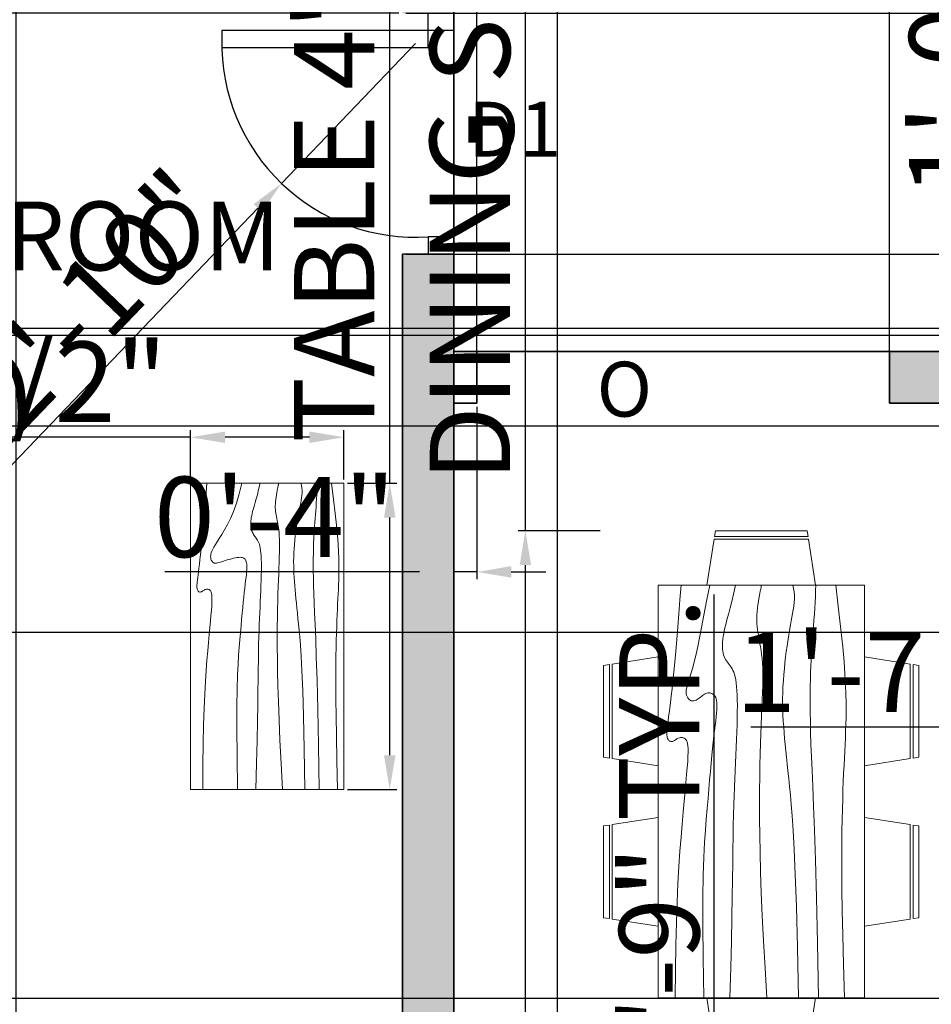
# Model space of a CAD drawing. Units: inches. Extents: x 2961 to 3748, y 1432 to 1961.
# Tile 3 of 9: x 3188 to 3348, y 1541 to 1713. Entities that reach past the tile are written whole.
import ezdxf
from ezdxf.enums import TextEntityAlignment as Align

# ---------------------------------------------------------------- set-up
doc = ezdxf.new("R2010")
doc.units = ezdxf.units.IN
for name, color, linetype, lineweight in [('A-ANNO-DIMS', 2, 'Continuous', 18), ('A-ANNO-TEXT', 7, 'Continuous', 18), ('A-AREA-IDEN', 7, 'Continuous', 18), ('A-DOOR', 3, 'Continuous', 25), ('A-FURN', 8, 'Continuous', 18), ('A-WALL', 7, 'Continuous', 35), ('A-WALL-PATT', 252, 'Continuous', 13)]:
    doc.layers.add(name, color=color, linetype=linetype, lineweight=lineweight)
doc.styles.get("Standard").update_dxf_attribs({"font": 'arial.ttf'})
doc.dimstyles.new('ISO-25', dxfattribs={"dimtxt": 14, "dimasz": 6, "dimexe": 1.25, "dimexo": 0.625, "dimtad": 1, "dimlunit": 3, "dimtxsty": 'Standard', "dimcen": 2.5, "dimadec": 0, "dimazin": 0, "dimtfac": 1, "dimtmove": 0, "dimatfit": 3, "dimfxl": 1, "dimarcsym": 0})

# ---------------------------------------------------------------- blocks, each defined once
blk = doc.blocks.new('Dining Set - 36 x 72 in.')
for p, q in [((-22, 27.5), (-22.1562, 26.50042)), ((-22, 27.5), (-6, 27.5)), ((-5.8437, 26.49966), (-6, 27.5)), ((6, 27.5), (5.8438, 26.50042)), ((6, 27.5), (22, 27.5)), ((22.1563, 26.49966), (22, 27.5)), ((-22.2343, 26.00059), (-23.4847, 17.99762)), ((-22.2304, 26), (-5.7608, 26)), ((-5.8416, 26.5), (-22.1534, 26.5)), ((-4.5152, 17.99762), (-5.7655, 25.99926)), ((5.7657, 26.00059), (4.5153, 17.99762)), ((5.7696, 26), (22.2392, 26)), ((22.1584, 26.5), (5.8466, 26.5)), ((23.4848, 17.99762), (22.2345, 25.99926)), ((36, 18), (-36, 18)), ((-36, 18), (-36, -18)), ((36, -18), (36, 18)), ((-44.0006, 8.23428), (-35.9976, 9.48474)), ((44.0006, 8.23428), (35.9976, 9.48474)), ((-45.5, 8), (-44.5004, 8.15617)), ((-45.5, 8), (-45.5, -8)), ((-44.5, -8.15843), (-44.5, 8.15338)), ((-44, 8.23041), (-44, -8.23915)), ((44, 8.23041), (44, -8.23915)), ((44.5, -8.15843), (44.5, 8.15338)), ((45.5, 8), (44.5005, 8.15617)), ((45.5, 8), (45.5, -8)), ((-44.4997, -8.15631), (-45.5, -8)), ((-35.9976, -9.48476), (-43.9993, -8.2345)), ((35.9976, -9.48476), (43.9993, -8.2345)), ((44.4997, -8.15631), (45.5, -8)), ((-36, -18), (36, -18)), ((-22.2343, -26.0006), (-23.4847, -17.99762)), ((-4.5152, -17.99762), (-5.7655, -25.99928)), ((5.7657, -26.0006), (4.5153, -17.99762)), ((23.4848, -17.99762), (22.2345, -25.99928)), ((-22.2304, -26), (-5.7608, -26)), ((-22, -27.5), (-22.1562, -26.50044)), ((-5.8416, -26.5), (-22.1534, -26.5)), ((-5.8437, -26.49967), (-6, -27.5)), ((5.7696, -26), (22.2392, -26)), ((6, -27.5), (5.8438, -26.50044)), ((22.1584, -26.5), (5.8466, -26.5)), ((22.1563, -26.49967), (22, -27.5)), ((-22, -27.5), (-6, -27.5)), ((6, -27.5), (22, -27.5))]:
    blk.add_line(p, q)
for points in [[(-36, 15), (-31.1772, 14.97754), (-26.8079, 14.91406), (-22.8538, 14.81543), (-19.276, 14.6875), (-16.0362, 14.53613), (-13.0957, 14.36718), (-10.4159, 14.18652), (-7.9583, 14), (-5.6904, 13.81315), (-3.6035, 13.63021), (-1.6954, 13.45508), (0.0365, 13.29166), (1.5945, 13.14388), (2.9811, 13.01562), (4.1988, 12.9108), (5.25, 12.83333), (6.1393, 12.78613), (6.8802, 12.76823), (7.4883, 12.77767), (7.9792, 12.8125), (8.3685, 12.87077), (8.6719, 12.95052), (8.9049, 13.0498), (9.0833, 13.16666), (9.2205, 13.29899), (9.3216, 13.44401), (9.3895, 13.59879), (9.4271, 13.76041), (9.4373, 13.92594), (9.4232, 14.09245), (9.3875, 14.257), (9.3333, 14.41666), (9.2638, 14.56917), (9.1836, 14.71484), (9.0975, 14.85465), (9.0104, 14.98958), (8.9272, 15.1206), (8.8529, 15.2487), (8.7922, 15.37483), (8.75, 15.5), (8.7305, 15.62467), (8.7344, 15.74739), (8.7617, 15.86621), (8.8125, 15.97916), (8.8867, 16.08431), (8.9844, 16.17968), (9.1055, 16.26334), (9.25, 16.33333), (9.4189, 16.38802), (9.6172, 16.42708), (9.8506, 16.45052), (10.125, 16.45833), (10.4463, 16.45052), (10.8203, 16.42708), (11.2529, 16.38802), (11.75, 16.33333), (12.3184, 16.26318), (12.9694, 16.17838), (13.7151, 16.07991), (14.5677, 15.96875), (15.5395, 15.84586), (16.6426, 15.71224), (17.8893, 15.56884), (19.2917, 15.41666), (20.859, 15.25667), (22.5879, 15.08984), (24.4721, 14.91715), (26.5052, 14.73958), (28.6809, 14.5581), (30.9929, 14.3737), (33.4347, 14.18733), (36, 14)], [(-36, 10), (-28.9766, 10.14274), (-23.1725, 10.20442), (-18.4241, 10.19775), (-14.5677, 10.13541), (-11.4399, 10.03011), (-8.877, 9.89453), (-6.7154, 9.74137), (-4.7917, 9.58333), (-2.9698, 9.43082), (-1.2246, 9.28515), (0.4415, 9.14534), (2.026, 9.01041), (3.5266, 8.87939), (4.9408, 8.7513), (6.266, 8.62516), (7.5, 8.5), (8.6411, 8.37549), (9.6914, 8.2539), (10.6538, 8.13818), (11.5312, 8.03125), (12.3267, 7.93603), (13.043, 7.85547), (13.6831, 7.79248), (14.25, 7.75), (14.7471, 7.7303), (15.1797, 7.73307), (15.5537, 7.75732), (15.875, 7.80208), (16.1494, 7.86637), (16.3828, 7.94922), (16.5811, 8.04964), (16.75, 8.16666), (16.8944, 8.29915), (17.0143, 8.44531), (17.1089, 8.60319), (17.1771, 8.77083), (17.218, 8.94629), (17.2305, 9.1276), (17.2137, 9.31282), (17.1667, 9.5), (17.0895, 9.6875), (16.987, 9.875), (16.8649, 10.0625), (16.7292, 10.25), (16.5856, 10.4375), (16.4401, 10.625), (16.2985, 10.8125), (16.1667, 11), (16.05, 11.18733), (15.9518, 11.3737), (15.8752, 11.5581), (15.8229, 11.73958), (15.798, 11.91715), (15.8034, 12.08984), (15.842, 12.25667), (15.9167, 12.41666), (16.0295, 12.56836), (16.1784, 12.70833), (16.3605, 12.83268), (16.5729, 12.9375), (16.8127, 13.01888), (17.0768, 13.07291), (17.3625, 13.0957), (17.6667, 13.08333), (17.9894, 13.03312), (18.3418, 12.94726), (18.7382, 12.82918), (19.1927, 12.68229), (19.7195, 12.51001), (20.3327, 12.31575), (21.0465, 12.10294), (21.875, 11.875), (22.8357, 11.63354), (23.959, 11.37304), (25.2786, 11.08618), (26.8282, 10.76562), (28.6414, 10.40405), (30.752, 9.99414), (33.1936, 9.52856), (36, 9)], [(-36, 5.5), (-30.7157, 5.3348), (-26.069, 5.20963), (-21.9946, 5.11767), (-18.4271, 5.05208), (-15.3009, 5.00602), (-12.5508, 4.97265), (-10.1112, 4.94515), (-7.9167, 4.91666), (-5.909, 4.88167), (-4.0586, 4.83984), (-2.3429, 4.79215), (-0.7396, 4.73958), (0.7739, 4.6831), (2.22, 4.6237), (3.6213, 4.56233), (5, 4.5), (6.373, 4.43782), (7.7344, 4.3776), (9.0723, 4.32129), (10.375, 4.27083), (11.6309, 4.22819), (12.8281, 4.19531), (13.9551, 4.17415), (15, 4.16666), (15.954, 4.17448), (16.819, 4.19791), (17.6001, 4.23698), (18.3021, 4.29166), (18.9299, 4.36198), (19.4883, 4.44791), (19.9823, 4.54948), (20.4167, 4.66666), (20.7969, 4.79899), (21.1302, 4.94401), (21.4245, 5.09879), (21.6875, 5.26041), (21.9271, 5.42594), (22.1511, 5.59245), (22.3672, 5.757), (22.5834, 5.91666), (22.8065, 6.06868), (23.0404, 6.21093), (23.2879, 6.34147), (23.5521, 6.45833), (23.8358, 6.55957), (24.142, 6.64323), (24.4735, 6.70735), (24.8334, 6.75), (25.2235, 6.76969), (25.642, 6.76692), (26.0858, 6.74267), (26.5521, 6.69791), (27.0379, 6.63362), (27.5404, 6.55078), (28.0565, 6.45036), (28.5834, 6.33333), (29.1242, 6.19987), (29.7071, 6.04687), (30.3661, 5.87044), (31.1354, 5.66666), (32.0493, 5.43164), (33.142, 5.16146), (34.4475, 4.85221), (36, 4.5)], [(-36, -1), (-30.7915, -0.6591), (-26.0195, -0.38216), (-21.6519, -0.16284), (-17.6563, 0.00521), (-14.0005, 0.12833), (-10.6523, 0.21289), (-7.5796, 0.26522), (-4.75, 0.29166), (-2.134, 0.29793), (0.2878, 0.28711), (2.5317, 0.26163), (4.6146, 0.22396), (6.5529, 0.17651), (8.3633, 0.12174), (10.0623, 0.06209), (11.6667, 0), (13.1899, -0.06201), (14.6341, -0.1211), (15.9982, -0.17432), (17.2813, -0.21875), (18.4823, -0.25147), (19.6003, -0.26953), (20.6343, -0.27002), (21.5834, -0.25), (22.4481, -0.20768), (23.2357, -0.14584), (23.9549, -0.06836), (24.6146, 0.02083), (25.2235, 0.11784), (25.7904, 0.21875), (26.3241, 0.31966), (26.8334, 0.41666), (27.3265, 0.50618), (27.8099, 0.58593), (28.2894, 0.65397), (28.7709, 0.70833), (29.2601, 0.74707), (29.763, 0.76823), (30.2855, 0.76985), (30.8334, 0.75), (31.4088, 0.70784), (31.9994, 0.64713), (32.589, 0.57275), (33.1615, 0.48958), (33.7008, 0.4025), (34.1908, 0.3164), (34.6153, 0.23616), (34.9584, 0.16666), (35.2099, 0.11165), (35.3848, 0.07031), (35.504, 0.04069), (35.5886, 0.02083), (35.6594, 0.00879), (35.7377, 0.0026), (35.8442, 0.00032), (36, 0)], [(-36, -6.5), (-27.1843, -6.31267), (-20.084, -6.1263), (-14.469, -5.9419), (-10.1094, -5.76042), (-6.7752, -5.58285), (-4.2363, -5.41016), (-2.2629, -5.24333), (-0.625, -5.08334), (0.8708, -4.93099), (2.2715, -4.78646), (3.5872, -4.64974), (4.8281, -4.52084), (6.0046, -4.39974), (7.127, -4.28646), (8.2053, -4.18099), (9.25, -4.08334), (10.2705, -3.99382), (11.2734, -3.91407), (12.2647, -3.84603), (13.25, -3.79167), (14.2354, -3.75293), (15.2266, -3.73177), (16.2295, -3.73015), (17.25, -3.75), (18.2912, -3.79248), (19.3451, -3.85547), (20.4009, -3.93604), (21.4479, -4.03125), (22.4754, -4.13819), (23.4727, -4.25391), (24.4289, -4.37549), (25.3334, -4.5), (26.1785, -4.62492), (26.9694, -4.74935), (27.7145, -4.87281), (28.4219, -4.99479), (29.1, -5.11483), (29.7572, -5.23242), (30.4016, -5.34709), (31.0417, -5.45834), (31.6837, -5.56437), (32.3262, -5.65821), (32.9658, -5.73153), (33.599, -5.77604), (34.2224, -5.78345), (34.8327, -5.74545), (35.4264, -5.65373), (36, -5.5)], [(-36, -10), (-26.4022, -9.81299), (-18.4675, -9.62891), (-11.9839, -9.45069), (-6.7396, -9.28125), (-2.5226, -9.12354), (0.8789, -8.98047), (3.6769, -8.85498), (6.0833, -8.75), (8.2767, -8.66765), (10.3021, -8.60677), (12.1712, -8.56543), (13.8958, -8.54167), (15.4876, -8.53353), (16.9583, -8.53907), (18.3197, -8.55632), (19.5834, -8.58334), (20.7616, -8.61841), (21.8685, -8.66081), (22.9188, -8.71004), (23.9271, -8.76563), (24.9081, -8.82707), (25.8763, -8.89388), (26.8465, -8.96558), (27.8334, -9.04167), (28.8474, -9.12118), (29.8828, -9.20117), (30.93, -9.27824), (31.9792, -9.34896), (33.0205, -9.40991), (34.0443, -9.45768), (35.0407, -9.48885), (36, -9.5)], [(-36, -14.5), (-30.0881, -14.33513), (-25.0332, -14.21224), (-20.7312, -14.12647), (-17.0781, -14.07292), (-13.97, -14.04671), (-11.3027, -14.04297), (-8.9724, -14.05681), (-6.875, -14.08334), (-4.9224, -14.11833), (-3.0905, -14.16016), (-1.3709, -14.20785), (0.2448, -14.26042), (1.7647, -14.3169), (3.1973, -14.3763), (4.5507, -14.43767), (5.8333, -14.5), (7.0554, -14.5621), (8.235, -14.62175), (9.3922, -14.67652), (10.5469, -14.72396), (11.7192, -14.76164), (12.929, -14.78711), (14.1965, -14.79794), (15.5417, -14.79167), (16.9933, -14.76424), (18.6152, -14.70508), (20.4804, -14.60197), (22.6615, -14.44271), (25.2312, -14.21509), (28.2624, -13.9069), (31.8277, -13.50594), (36, -13)]]:
    blk.add_lwpolyline(points)
blk = doc.blocks.new('Table - Rectangular Woodgrain 60 x 30 in.')
for p, q in [((0, 0), (0, -30)), ((60, 0), (0, 0)), ((60, -30), (60, 0)), ((0, -30), (60, -30))]:
    blk.add_line(p, q)
for points in [[(0, -2.4), (4.8155, -2.418), (9.0302, -2.4688), (12.709, -2.5477), (15.9167, -2.65), (18.7181, -2.7711), (21.1781, -2.9063), (23.3616, -3.0508), (25.3333, -3.2), (27.1477, -3.3495), (28.8172, -3.4958), (30.3437, -3.636), (31.7291, -3.7667), (32.9756, -3.8849), (34.0849, -3.9875), (35.059, -4.0714), (35.9, -4.1334), (36.6114, -4.1711), (37.2041, -4.1854), (37.6906, -4.1779), (38.0833, -4.15), (38.3948, -4.1034), (38.6375, -4.0396), (38.8239, -3.9602), (38.9666, -3.8667), (39.0764, -3.7608), (39.1573, -3.6448), (39.2116, -3.521), (39.2416, -3.3917), (39.2498, -3.2593), (39.2385, -3.1261), (39.21, -2.9944), (39.1666, -2.8667), (39.111, -2.7447), (39.0468, -2.6281), (38.978, -2.5163), (38.9083, -2.4083), (38.8418, -2.3035), (38.7823, -2.201), (38.7337, -2.1001), (38.7, -2), (38.6844, -1.9003), (38.6875, -1.8021), (38.7094, -1.707), (38.75, -1.6167), (38.8094, -1.5326), (38.8875, -1.4563), (38.9844, -1.3893), (39.1, -1.3333), (39.2351, -1.2896), (39.3937, -1.2583), (39.5804, -1.2396), (39.8, -1.2333), (40.057, -1.2396), (40.3562, -1.2583), (40.7023, -1.2896), (41.1, -1.3333), (41.5547, -1.3895), (42.0755, -1.4573), (42.6721, -1.5361), (43.3542, -1.625), (44.1316, -1.7233), (45.014, -1.8302), (46.0114, -1.9449), (47.1333, -2.0667), (48.3862, -2.1947), (49.7625, -2.3281), (51.2513, -2.4663), (52.8416, -2.6083), (54.5226, -2.7535), (56.2833, -2.9011), (58.1127, -3.0501), (60, -3.2)], [(0, -9.2), (6.5759, -9.0858), (11.9385, -9.0365), (16.2527, -9.0418), (19.6833, -9.0917), (22.3952, -9.1759), (24.5531, -9.2844), (26.322, -9.4069), (27.8666, -9.5333), (29.3241, -9.6553), (30.7203, -9.7719), (32.0532, -9.8837), (33.3208, -9.9917), (34.5213, -10.0965), (35.6526, -10.199), (36.7128, -10.2999), (37.7, -10.4), (38.6129, -10.4996), (39.4531, -10.5969), (40.223, -10.6895), (40.925, -10.775), (41.5613, -10.8512), (42.1344, -10.9156), (42.6465, -10.966), (43.1, -11), (43.4976, -11.0158), (43.8437, -11.0136), (44.143, -10.9942), (44.4, -10.9583), (44.6195, -10.9069), (44.8062, -10.8406), (44.9648, -10.7603), (45.1, -10.6667), (45.2155, -10.5598), (45.3114, -10.4365), (45.3871, -10.2929), (45.4416, -10.125), (45.4743, -9.929), (45.4844, -9.7011), (45.4709, -9.4371), (45.4333, -9.1333), (45.3716, -8.7883), (45.2896, -8.4104), (45.1919, -8.0107), (45.0833, -7.6), (44.9685, -7.1893), (44.8521, -6.7896), (44.7388, -6.4117), (44.6333, -6.0667), (44.54, -5.7628), (44.4614, -5.4979), (44.4001, -5.2675), (44.3583, -5.0667), (44.3384, -4.8909), (44.3427, -4.7354), (44.3736, -4.5956), (44.4333, -4.4667), (44.5236, -4.3453), (44.6427, -4.2333), (44.7884, -4.1339), (44.9583, -4.05), (45.1501, -3.9849), (45.3614, -3.9417), (45.59, -3.9234), (45.8333, -3.9333), (46.0915, -3.9749), (46.3734, -4.0531), (46.6906, -4.1736), (47.0542, -4.3417), (47.4756, -4.5629), (47.9661, -4.8427), (48.5372, -5.1866), (49.2, -5.6), (49.9676, -6.0844), (50.8594, -6.625), (51.8965, -7.2031), (53.1, -7.8), (54.491, -8.3969), (56.0906, -8.975), (57.9199, -9.5156), (60, -10)], [(0, -12.8), (5.1847, -12.9322), (9.6213, -13.0323), (13.3963, -13.1059), (16.5958, -13.1583), (19.3063, -13.1952), (21.614, -13.2219), (23.6054, -13.2439), (25.3666, -13.2667), (26.9728, -13.2947), (28.4531, -13.3281), (29.8256, -13.3663), (31.1083, -13.4083), (32.3191, -13.4535), (33.476, -13.501), (34.597, -13.5501), (35.7, -13.6), (36.7984, -13.6497), (37.8875, -13.6979), (38.9578, -13.743), (40, -13.7833), (41.0047, -13.8174), (41.9625, -13.8438), (42.864, -13.8607), (43.7, -13.8667), (44.4631, -13.8604), (45.1552, -13.8417), (45.7801, -13.8104), (46.3416, -13.7667), (46.8439, -13.7104), (47.2906, -13.6417), (47.6858, -13.5604), (48.0333, -13.4667), (48.3375, -13.3608), (48.6042, -13.2448), (48.8396, -13.121), (49.05, -12.9917), (49.2417, -12.8593), (49.4208, -12.7261), (49.5937, -12.5944), (49.7667, -12.4667), (49.9452, -12.3451), (50.1323, -12.2313), (50.3303, -12.1268), (50.5416, -12.0333), (50.7686, -11.9524), (51.0135, -11.8854), (51.2788, -11.8341), (51.5666, -11.8), (51.8785, -11.7843), (52.2116, -11.7865), (52.562, -11.8059), (52.926, -11.8417), (53.2998, -11.8931), (53.6795, -11.9594), (54.0614, -12.0397), (54.4416, -12.1333), (54.8223, -12.2401), (55.2293, -12.3625), (55.6942, -12.5037), (56.2489, -12.6667), (56.9251, -12.8547), (57.7545, -13.0708), (58.7689, -13.3182), (60, -13.6)], [(0, -18), (5.124, -17.7273), (9.6609, -17.5057), (13.6705, -17.3303), (17.2125, -17.1958), (20.3467, -17.0973), (23.1328, -17.0297), (25.6307, -16.9878), (27.9, -16.9667), (29.9928, -16.9617), (31.9302, -16.9703), (33.7254, -16.9907), (35.3917, -17.0208), (36.9423, -17.0588), (38.3906, -17.1026), (39.7499, -17.1503), (41.0333, -17.2), (42.2519, -17.2496), (43.4073, -17.2969), (44.4986, -17.3395), (45.525, -17.375), (46.4858, -17.4012), (47.3802, -17.4156), (48.2074, -17.416), (48.9667, -17.4), (49.6583, -17.3662), (50.2872, -17.3167), (50.8595, -17.2547), (51.3812, -17.1833), (51.8584, -17.1057), (52.2971, -17.025), (52.7034, -16.9443), (53.0833, -16.8667), (53.443, -16.7951), (53.789, -16.7313), (54.128, -16.6768), (54.4666, -16.6334), (54.8115, -16.6024), (55.1693, -16.5854), (55.5465, -16.5841), (55.95, -16.6), (56.3828, -16.6337), (56.8346, -16.6823), (57.2915, -16.7418), (57.7396, -16.8084), (58.165, -16.878), (58.5539, -16.9469), (58.8924, -17.0111), (59.1666, -17.0667), (59.3679, -17.1107), (59.5078, -17.1438), (59.6032, -17.1675), (59.6708, -17.1833), (59.7275, -17.193), (59.7901, -17.1979), (59.8753, -17.1998), (60, -17.2)], [(0, -22.4), (8.0098, -22.2501), (14.4094, -22.1011), (19.4168, -21.9535), (23.25, -21.8083), (26.1269, -21.6663), (28.2656, -21.5281), (29.884, -21.3947), (31.2, -21.2667), (32.3967, -21.1448), (33.5172, -21.0292), (34.5697, -20.9198), (35.5625, -20.8167), (36.5037, -20.7198), (37.4015, -20.6292), (38.2642, -20.5448), (39.1, -20.4667), (39.9164, -20.3951), (40.7187, -20.3313), (41.5117, -20.2768), (42.3, -20.2333), (43.0883, -20.2024), (43.8812, -20.1854), (44.6836, -20.1841), (45.5, -20.2), (46.3328, -20.234), (47.1747, -20.2844), (48.0163, -20.3488), (48.8479, -20.425), (49.66, -20.5106), (50.4429, -20.6031), (51.1872, -20.7004), (51.8833, -20.8), (52.5246, -20.8999), (53.1166, -20.9995), (53.6681, -21.0983), (54.1875, -21.1958), (54.6834, -21.2919), (55.1646, -21.3859), (55.6394, -21.4777), (56.1167, -21.5667), (56.6028, -21.6515), (57.0961, -21.7266), (57.5929, -21.7852), (58.0896, -21.8208), (58.5823, -21.8268), (59.0674, -21.7964), (59.5412, -21.723), (60, -21.6)], [(0, -25.2), (8.6355, -25.0504), (15.7026, -24.9031), (21.4049, -24.7606), (25.9458, -24.625), (29.529, -24.4988), (32.3578, -24.3844), (34.6359, -24.284), (36.5667, -24.2), (38.3213, -24.1341), (39.9417, -24.0854), (41.437, -24.0523), (42.8167, -24.0333), (44.0901, -24.0268), (45.2667, -24.0313), (46.3557, -24.0451), (47.3667, -24.0667), (48.309, -24.0947), (49.1928, -24.1287), (50.0284, -24.168), (50.826, -24.2125), (51.5959, -24.2617), (52.3483, -24.3151), (53.0935, -24.3725), (53.8417, -24.4334), (54.6009, -24.497), (55.3699, -24.561), (56.1454, -24.6226), (56.9239, -24.6792), (57.7021, -24.7279), (58.4764, -24.7662), (59.2435, -24.7911), (60, -24.8)], [(0, -28.8), (5.6867, -28.6681), (10.45, -28.5698), (14.407, -28.5012), (17.675, -28.4584), (20.3711, -28.4374), (22.6125, -28.4344), (24.5164, -28.4455), (26.2, -28.4667), (27.762, -28.4947), (29.2276, -28.5281), (30.6033, -28.5663), (31.8958, -28.6084), (33.1118, -28.6535), (34.2578, -28.7011), (35.3405, -28.7501), (36.3666, -28.8), (37.3443, -28.8497), (38.288, -28.8974), (39.2137, -28.9412), (40.1375, -28.9792), (41.0753, -29.0093), (42.0432, -29.0297), (43.0572, -29.0384), (44.1333, -29.0333), (45.2936, -29.0114), (46.5843, -28.9641), (48.0579, -28.8816), (49.7666, -28.7542), (51.7629, -28.5721), (54.0989, -28.3255), (56.8272, -28.0048), (60, -27.6)]]:
    blk.add_lwpolyline(points)
blk = doc.blocks.new('*D21')
at = {"layer": 'A-ANNO-DIMS', "color": 0, "lineweight": -2, "transparency": 16777216}
for p, q in [((3309.67, 1519.64), (3309.67, 1612.23)), ((3304.89, 1513.64), (3310.92, 1513.64)), ((3309.67, 1504.64), (3309.67, 1513.64)), ((3304.89, 1504.64), (3310.92, 1504.64)), ((3309.67, 1498.64), (3309.67, 1492.64))]:
    blk.add_line(p, q, dxfattribs=at)
at = {"layer": 'A-ANNO-DIMS', "color": 0, "transparency": 16777216}
for points in [[(3308.67, 1519.64), (3310.67, 1519.64), (3309.67, 1513.64)], [(3308.67, 1498.64), (3310.67, 1498.64), (3309.67, 1504.64)]]:
    blk.add_solid(points, dxfattribs=at)
at = {"layer": 'Defpoints', "color": 0, "transparency": 16777216}
for p in [(3304.27, 1513.64), (3309.67, 1513.64), (3304.27, 1504.64)]:
    blk.add_point(p, dxfattribs=at)
at = {"layer": 'A-ANNO-DIMS', "color": 0, "transparency": 16777216, "insert": (3301.89, 1568.93), "char_height": 14, "attachment_point": 5, "rotation": 90}
blk.add_mtext('0\'-9" TYP.', dxfattribs=at)
blk = doc.blocks.new('*D28')
at = {"layer": 'A-ANNO-DIMS', "color": 0, "lineweight": -2, "transparency": 16777216}
for p, q in [((3253.06, 1631.67), (3253.06, 1776.5)), ((3245.67, 1631.67), (3254.31, 1631.67)), ((3253.06, 1584.22), (3253.06, 1625.67)), ((3245.67, 1578.22), (3254.31, 1578.22))]:
    blk.add_line(p, q, dxfattribs=at)
at = {"layer": 'A-ANNO-DIMS', "color": 0, "transparency": 16777216}
for points in [[(3252.06, 1625.67), (3254.06, 1625.67), (3253.06, 1631.67)], [(3252.06, 1584.22), (3254.06, 1584.22), (3253.06, 1578.22)]]:
    blk.add_solid(points, dxfattribs=at)
at = {"layer": 'Defpoints', "color": 0, "transparency": 16777216}
for p in [(3245.04, 1631.67), (3253.06, 1631.67), (3245.04, 1578.22)]:
    blk.add_point(p, dxfattribs=at)
at = {"layer": 'A-ANNO-DIMS', "color": 0, "transparency": 16777216, "insert": (3245.19, 1707.08), "char_height": 14, "attachment_point": 5, "rotation": 90}
blk.add_mtext('TABLE 4\'-5 1/2"', dxfattribs=at)
blk = doc.blocks.new('*D29')
at = {"layer": 'A-ANNO-DIMS', "color": 0, "lineweight": -2, "transparency": 16777216}
for p, q in [((3218.32, 1632.29), (3218.32, 1640.93)), ((3245.04, 1632.29), (3245.04, 1640.93)), ((3218.32, 1639.68), (3140.99, 1639.68)), ((3239.04, 1639.68), (3224.32, 1639.68))]:
    blk.add_line(p, q, dxfattribs=at)
at = {"layer": 'A-ANNO-DIMS', "color": 0, "transparency": 16777216}
for points in [[(3224.32, 1640.68), (3224.32, 1638.68), (3218.32, 1639.68)], [(3239.04, 1640.68), (3239.04, 1638.68), (3245.04, 1639.68)]]:
    blk.add_solid(points, dxfattribs=at)
at = {"layer": 'Defpoints', "color": 0, "transparency": 16777216}
for p in [(3218.32, 1639.68), (3218.32, 1631.67), (3245.04, 1631.67)]:
    blk.add_point(p, dxfattribs=at)
at = {"layer": 'A-ANNO-DIMS', "color": 0, "transparency": 16777216, "insert": (3176.66, 1647.55), "char_height": 14, "attachment_point": 5}
blk.add_mtext('2\'-2 1/2"', dxfattribs=at)
blk = doc.blocks.new('*D41')
at = {"layer": 'A-ANNO-DIMS', "color": 0, "lineweight": -2, "transparency": 16777216}
for p, q in [((3391.84, 1586.08), (3391.84, 1590.35)), ((3411.44, 1586.08), (3411.44, 1590.35)), ((3391.84, 1589.1), (3316.07, 1589.1)), ((3405.44, 1589.1), (3397.84, 1589.1))]:
    blk.add_line(p, q, dxfattribs=at)
at = {"layer": 'A-ANNO-DIMS', "color": 0, "transparency": 16777216}
for points in [[(3397.84, 1590.1), (3397.84, 1588.1), (3391.84, 1589.1)], [(3405.44, 1590.1), (3405.44, 1588.1), (3411.44, 1589.1)]]:
    blk.add_solid(points, dxfattribs=at)
at = {"layer": 'Defpoints', "color": 0, "transparency": 16777216}
for p in [(3391.84, 1589.1), (3391.84, 1585.45), (3411.44, 1585.45)]:
    blk.add_point(p, dxfattribs=at)
at = {"layer": 'A-ANNO-DIMS', "color": 0, "transparency": 16777216, "insert": (3350.95, 1596.96), "char_height": 14, "attachment_point": 5}
blk.add_mtext('1\'-7 1/2"', dxfattribs=at)
blk = doc.blocks.new('*D44')
at = {"layer": 'A-ANNO-DIMS', "color": 0, "lineweight": -2, "transparency": 16777216}
for p, q in [((3276.73, 1623.38), (3276.73, 1784.51)), ((3289.75, 1623.38), (3275.48, 1623.38)), ((3276.73, 1538.38), (3276.73, 1617.38)), ((3289.75, 1532.38), (3275.48, 1532.38))]:
    blk.add_line(p, q, dxfattribs=at)
at = {"layer": 'A-ANNO-DIMS', "color": 0, "transparency": 16777216}
for points in [[(3275.73, 1617.38), (3277.73, 1617.38), (3276.73, 1623.38)], [(3275.73, 1538.38), (3277.73, 1538.38), (3276.73, 1532.38)]]:
    blk.add_solid(points, dxfattribs=at)
at = {"layer": 'Defpoints', "color": 0, "transparency": 16777216}
for p in [(3276.73, 1623.38), (3290.38, 1623.38), (3290.38, 1532.38)]:
    blk.add_point(p, dxfattribs=at)
at = {"layer": 'A-ANNO-DIMS', "color": 0, "transparency": 16777216, "insert": (3268.87, 1706.94), "char_height": 14, "attachment_point": 5, "rotation": 90}
blk.add_mtext('DINING SET 7\'-7"', dxfattribs=at)
blk = doc.blocks.new('*D52')
at = {"layer": 'A-ANNO-DIMS', "color": 0, "lineweight": -2, "transparency": 16777216}
for p, q in [((3360.27, 1678.21), (3360.27, 1721.36)), ((3389.1, 1672.21), (3359.02, 1672.21)), ((3360.27, 1660.05), (3360.27, 1672.21)), ((3389.1, 1660.05), (3359.02, 1660.05)), ((3360.27, 1654.05), (3360.27, 1648.05))]:
    blk.add_line(p, q, dxfattribs=at)
at = {"layer": 'A-ANNO-DIMS', "color": 0, "transparency": 16777216}
for points in [[(3359.27, 1678.21), (3361.27, 1678.21), (3360.27, 1672.21)], [(3359.27, 1654.05), (3361.27, 1654.05), (3360.27, 1660.05)]]:
    blk.add_solid(points, dxfattribs=at)
at = {"layer": 'Defpoints', "color": 0, "transparency": 16777216}
for p in [(3360.27, 1672.21), (3389.72, 1672.21), (3389.72, 1660.05)]:
    blk.add_point(p, dxfattribs=at)
at = {"layer": 'A-ANNO-DIMS', "color": 0, "transparency": 16777216, "insert": (3352.5, 1702.78), "char_height": 14, "attachment_point": 5, "rotation": 90}
blk.add_mtext('1\'-0"', dxfattribs=at)
blk = doc.blocks.new('*D53')
at = {"layer": 'A-ANNO-DIMS', "color": 0, "lineweight": -2, "transparency": 16777216}
for p, q in [((3123.27, 1855.01), (3123.27, 1473.94)), ((3187.8, 1855.01), (3187.8, 1473.94)), ((3129.27, 1475.19), (3181.8, 1475.19)), ((3187.8, 1475.19), (3264.89, 1475.19))]:
    blk.add_line(p, q, dxfattribs=at)
at = {"layer": 'A-ANNO-DIMS', "color": 0, "transparency": 16777216}
for points in [[(3129.27, 1476.19), (3129.27, 1474.19), (3123.27, 1475.19)], [(3181.8, 1476.19), (3181.8, 1474.19), (3187.8, 1475.19)]]:
    blk.add_solid(points, dxfattribs=at)
at = {"layer": 'Defpoints', "color": 0, "transparency": 16777216}
for p in [(3123.27, 1855.64), (3187.8, 1855.64), (3187.8, 1475.19)]:
    blk.add_point(p, dxfattribs=at)
at = {"layer": 'A-ANNO-DIMS', "color": 0, "transparency": 16777216, "insert": (3229.35, 1483.05), "char_height": 14, "attachment_point": 5}
blk.add_mtext('5\'-4 1/2"', dxfattribs=at)
blk = doc.blocks.new('*D68')
at = {"layer": 'A-ANNO-DIMS', "color": 0, "lineweight": -2, "transparency": 16777216}
for p, q in [((3024.82, 1658.64), (3024.82, 1701.79)), ((3509.64, 1658.64), (3023.57, 1658.64)), ((3024.82, 1647.64), (3024.82, 1652.64)), ((3509.64, 1641.64), (3023.57, 1641.64))]:
    blk.add_line(p, q, dxfattribs=at)
at = {"layer": 'A-ANNO-DIMS', "color": 0, "transparency": 16777216}
for points in [[(3023.82, 1652.64), (3025.82, 1652.64), (3024.82, 1658.64)], [(3023.82, 1647.64), (3025.82, 1647.64), (3024.82, 1641.64)]]:
    blk.add_solid(points, dxfattribs=at)
at = {"layer": 'Defpoints', "color": 0, "transparency": 16777216}
for p in [(3024.82, 1658.64), (3510.27, 1658.64), (3510.27, 1641.64)]:
    blk.add_point(p, dxfattribs=at)
at = {"layer": 'A-ANNO-DIMS', "color": 0, "transparency": 16777216, "insert": (3017.04, 1683.21), "char_height": 14, "attachment_point": 5, "rotation": 90}
blk.add_mtext('1\'-5"', dxfattribs=at)
blk = doc.blocks.new('*D69')
at = {"layer": 'A-ANNO-DIMS', "color": 0, "lineweight": -2, "transparency": 16777216}
for p, q in [((3268.27, 1646.26), (3268.27, 1933.63)), ((3274.27, 1932.38), (3334.27, 1932.38)), ((3340.27, 1646.26), (3340.27, 1933.63))]:
    blk.add_line(p, q, dxfattribs=at)
at = {"layer": 'A-ANNO-DIMS', "color": 0, "transparency": 16777216}
for points in [[(3274.27, 1933.38), (3274.27, 1931.38), (3268.27, 1932.38)], [(3334.27, 1933.38), (3334.27, 1931.38), (3340.27, 1932.38)]]:
    blk.add_solid(points, dxfattribs=at)
at = {"layer": 'Defpoints', "color": 0, "transparency": 16777216}
for p in [(3340.27, 1932.38), (3268.27, 1645.64), (3340.27, 1645.64)]:
    blk.add_point(p, dxfattribs=at)
at = {"layer": 'A-ANNO-DIMS', "color": 0, "transparency": 16777216, "insert": (3304.27, 1940.15), "char_height": 14, "attachment_point": 5}
blk.add_mtext('6\'-0"', dxfattribs=at)
blk = doc.blocks.new('*D70')
at = {"layer": 'A-ANNO-DIMS', "color": 0, "lineweight": -2, "transparency": 16777216}
for p, q in [((3024.82, 1641.64), (3024.82, 1686.09)), ((3383.64, 1641.64), (3023.57, 1641.64)), ((3024.82, 1611.64), (3024.82, 1635.64)), ((3383.64, 1605.64), (3023.57, 1605.64))]:
    blk.add_line(p, q, dxfattribs=at)
at = {"layer": 'A-ANNO-DIMS', "color": 0, "transparency": 16777216}
for points in [[(3023.82, 1635.64), (3025.82, 1635.64), (3024.82, 1641.64)], [(3023.82, 1611.64), (3025.82, 1611.64), (3024.82, 1605.64)]]:
    blk.add_solid(points, dxfattribs=at)
at = {"layer": 'Defpoints', "color": 0, "transparency": 16777216}
for p in [(3024.82, 1641.64), (3384.27, 1641.64), (3384.27, 1605.64)]:
    blk.add_point(p, dxfattribs=at)
at = {"layer": 'A-ANNO-DIMS', "color": 0, "transparency": 16777216, "insert": (3017.04, 1666.87), "char_height": 14, "attachment_point": 5, "rotation": 90}
blk.add_mtext('3\'-0"', dxfattribs=at)
blk = doc.blocks.new('*D72')
at = {"layer": 'A-ANNO-DIMS', "color": 0, "lineweight": -2, "transparency": 16777216}
for p, q in [((3255.89, 1713.64), (3633.97, 1713.64)), ((3632.72, 1677.64), (3632.72, 1707.64)), ((3255.89, 1671.64), (3633.97, 1671.64))]:
    blk.add_line(p, q, dxfattribs=at)
at = {"layer": 'A-ANNO-DIMS', "color": 0, "transparency": 16777216}
for points in [[(3631.72, 1707.64), (3633.72, 1707.64), (3632.72, 1713.64)], [(3631.72, 1677.64), (3633.72, 1677.64), (3632.72, 1671.64)]]:
    blk.add_solid(points, dxfattribs=at)
at = {"layer": 'Defpoints', "color": 0, "transparency": 16777216}
for p in [(3255.27, 1713.64), (3632.72, 1713.64), (3255.27, 1671.64)]:
    blk.add_point(p, dxfattribs=at)
at = {"layer": 'A-ANNO-DIMS', "color": 0, "transparency": 16777216, "insert": (3624.94, 1692.64), "char_height": 14, "attachment_point": 5, "rotation": 90}
blk.add_mtext('3\'-6"', dxfattribs=at)
blk = doc.blocks.new('*D75')
at = {"layer": 'A-ANNO-DIMS', "color": 0, "lineweight": -2, "transparency": 16777216}
for p, q in [((3024.82, 1723.64), (3024.82, 1729.64)), ((3254.64, 1717.64), (3023.57, 1717.64)), ((3024.82, 1717.64), (3024.82, 1713.64)), ((3254.64, 1713.64), (3023.57, 1713.64)), ((3024.82, 1707.64), (3024.82, 1663.17))]:
    blk.add_line(p, q, dxfattribs=at)
at = {"layer": 'A-ANNO-DIMS', "color": 0, "transparency": 16777216}
for points in [[(3023.82, 1723.64), (3025.82, 1723.64), (3024.82, 1717.64)], [(3023.82, 1707.64), (3025.82, 1707.64), (3024.82, 1713.64)]]:
    blk.add_solid(points, dxfattribs=at)
at = {"layer": 'Defpoints', "color": 0, "transparency": 16777216}
for p in [(3255.27, 1717.64), (3024.82, 1713.64), (3255.27, 1713.64)]:
    blk.add_point(p, dxfattribs=at)
at = {"layer": 'A-ANNO-DIMS', "color": 0, "transparency": 16777216, "insert": (3017.04, 1682.41), "char_height": 14, "attachment_point": 5, "rotation": 90}
blk.add_mtext('0\'-4"', dxfattribs=at)
blk = doc.blocks.new('*D77')
at = {"layer": 'A-ANNO-DIMS', "color": 0, "lineweight": -2, "transparency": 16777216}
for p, q in [((3264.27, 1775.91), (3264.27, 1473.94)), ((3282.27, 1775.91), (3282.27, 1473.94)), ((3270.27, 1475.19), (3276.27, 1475.19)), ((3282.27, 1475.19), (3325.41, 1475.19))]:
    blk.add_line(p, q, dxfattribs=at)
at = {"layer": 'A-ANNO-DIMS', "color": 0, "transparency": 16777216}
for points in [[(3270.27, 1476.19), (3270.27, 1474.19), (3264.27, 1475.19)], [(3276.27, 1476.19), (3276.27, 1474.19), (3282.27, 1475.19)]]:
    blk.add_solid(points, dxfattribs=at)
at = {"layer": 'Defpoints', "color": 0, "transparency": 16777216}
for p in [(3264.27, 1776.53), (3282.27, 1776.53), (3282.27, 1475.19)]:
    blk.add_point(p, dxfattribs=at)
at = {"layer": 'A-ANNO-DIMS', "color": 0, "transparency": 16777216, "insert": (3306.84, 1482.96), "char_height": 14, "attachment_point": 5}
blk.add_mtext('1\'-6"', dxfattribs=at)
blk = doc.blocks.new('*D81')
at = {"layer": 'A-ANNO-DIMS', "color": 0, "lineweight": -2, "transparency": 16777216}
for p, q in [((3063.89, 1657.48), (3633.97, 1657.48)), ((3632.72, 1547.87), (3632.72, 1651.48)), ((3063.89, 1541.87), (3633.97, 1541.87))]:
    blk.add_line(p, q, dxfattribs=at)
at = {"layer": 'A-ANNO-DIMS', "color": 0, "transparency": 16777216}
for points in [[(3631.72, 1651.48), (3633.72, 1651.48), (3632.72, 1657.48)], [(3631.72, 1547.87), (3633.72, 1547.87), (3632.72, 1541.87)]]:
    blk.add_solid(points, dxfattribs=at)
at = {"layer": 'Defpoints', "color": 0, "transparency": 16777216}
for p in [(3063.27, 1657.48), (3632.72, 1657.48), (3063.27, 1541.87)]:
    blk.add_point(p, dxfattribs=at)
at = {"layer": 'A-ANNO-DIMS', "color": 0, "transparency": 16777216, "insert": (3624.85, 1599.67), "char_height": 14, "attachment_point": 5, "rotation": 90}
blk.add_mtext('9\'-7 1/2"', dxfattribs=at)
blk = doc.blocks.new('*D84')
at = {"layer": 'A-ANNO-DIMS', "color": 0, "lineweight": -2, "transparency": 16777216}
for p, q in [((3123.27, 1855.01), (3123.27, 1473.94)), ((3137.88, 1855.01), (3137.88, 1473.94)), ((3129.27, 1475.19), (3131.88, 1475.19)), ((3137.88, 1475.19), (3213.65, 1475.19))]:
    blk.add_line(p, q, dxfattribs=at)
at = {"layer": 'A-ANNO-DIMS', "color": 0, "transparency": 16777216}
for points in [[(3129.27, 1476.19), (3129.27, 1474.19), (3123.27, 1475.19)], [(3131.88, 1476.19), (3131.88, 1474.19), (3137.88, 1475.19)]]:
    blk.add_solid(points, dxfattribs=at)
at = {"layer": 'Defpoints', "color": 0, "transparency": 16777216}
for p in [(3123.27, 1855.64), (3137.88, 1855.64), (3137.88, 1475.19)]:
    blk.add_point(p, dxfattribs=at)
at = {"layer": 'A-ANNO-DIMS', "color": 0, "transparency": 16777216, "insert": (3178.76, 1483.05), "char_height": 14, "attachment_point": 5}
blk.add_mtext('1\'-2 1/2"', dxfattribs=at)
blk = doc.blocks.new('*D89')
at = {"layer": 'A-ANNO-DIMS', "color": 0, "lineweight": -2, "transparency": 16777216}
for p, q in [((3264.27, 1645.01), (3264.27, 1614.94)), ((3268.27, 1645.01), (3268.27, 1614.94)), ((3258.27, 1616.19), (3213.8, 1616.19)), ((3268.27, 1616.19), (3264.27, 1616.19)), ((3274.27, 1616.19), (3280.27, 1616.19))]:
    blk.add_line(p, q, dxfattribs=at)
at = {"layer": 'A-ANNO-DIMS', "color": 0, "transparency": 16777216}
for points in [[(3258.27, 1617.19), (3258.27, 1615.19), (3264.27, 1616.19)], [(3274.27, 1617.19), (3274.27, 1615.19), (3268.27, 1616.19)]]:
    blk.add_solid(points, dxfattribs=at)
at = {"layer": 'Defpoints', "color": 0, "transparency": 16777216}
for p in [(3264.27, 1645.64), (3268.27, 1645.64), (3264.27, 1616.19)]:
    blk.add_point(p, dxfattribs=at)
at = {"layer": 'A-ANNO-DIMS', "color": 0, "transparency": 16777216, "insert": (3233.03, 1623.96), "char_height": 14, "attachment_point": 5}
blk.add_mtext('0\'-4"', dxfattribs=at)
blk = doc.blocks.new('*D93')
at = {"layer": 'A-ANNO-DIMS', "color": 0, "lineweight": -2, "transparency": 16777216}
for p, q in [((3257.58, 1708.39), (3234.18, 1683.97)), ((3182.46, 1630.01), (3230.03, 1679.64))]:
    blk.add_line(p, q, dxfattribs=at)
at = {"layer": 'A-ANNO-DIMS', "color": 0, "transparency": 16777216}
blk.add_solid([(3229.31, 1680.33), (3230.75, 1678.95), (3234.18, 1683.97)], dxfattribs=at)
at = {"layer": 'Defpoints', "color": 0, "transparency": 16777216}
for p in [(3257.58, 1708.39), (3234.18, 1683.97)]:
    blk.add_point(p, dxfattribs=at)
at = {"layer": 'A-ANNO-DIMS', "color": 0, "transparency": 16777216, "insert": (3198.56, 1658.04), "char_height": 14, "attachment_point": 5, "rotation": 46.2188}
blk.add_mtext('R2\'-10"', dxfattribs=at)

msp = doc.modelspace()

# ---------------------------------------------------------------- hatches: boundary and pattern name
at = {"layer": 'A-WALL-PATT'}
h = msp.add_hatch(color=256, dxfattribs=at)
h.set_gradient(color1=(41, 49, 137), color2=(41, 49, 137), tint=1)
h.paths.add_polyline_path([(3255.267, 1671.639), (3255.267, 1513.639), (3251.267, 1513.639), (3251.267, 1504.639), (3268.267, 1504.639), (3268.267, 1513.639), (3264.267, 1513.639), (3264.267, 1671.639), (3259.767, 1671.639)])
h.paths.add_polyline_path([(3063.267, 1513.639), (3063.267, 1677.639), (3054.267, 1677.639), (3054.267, 1504.639), (3215.267, 1504.639), (3215.267, 1513.639)])
h.paths.add_polyline_path([(3304.267, 1513.639), (3304.267, 1504.639), (3456.267, 1504.639), (3456.267, 1513.639), (3390.267, 1513.639), (3390.267, 1605.639), (3384.267, 1605.639), (3384.267, 1513.639)])
h.paths.add_polyline_path([(3510.267, 1605.639), (3510.267, 1513.639), (3492.267, 1513.639), (3492.267, 1504.639), (3546.267, 1504.639), (3546.267, 1513.639), (3519.267, 1513.639), (3519.267, 1605.639)])
h.paths.add_polyline_path([(3340.267, 1654.639), (3340.267, 1645.639), (3510.267, 1645.639), (3510.267, 1641.639), (3519.267, 1641.639), (3519.267, 1658.639), (3510.267, 1658.639), (3510.267, 1654.639)])
h.paths.add_polyline_path([(3223.801, 1864.639), (3223.801, 1855.639), (3255.267, 1855.639), (3255.267, 1772.534), (3264.267, 1772.534), (3264.267, 1855.639), (3303.267, 1855.639), (3303.267, 1864.639)])
h.paths.add_polyline_path([(3339.267, 1864.639), (3339.267, 1855.639), (3435.267, 1855.639), (3435.267, 1864.639)])
h.paths.add_polyline_path([(3471.267, 1864.639), (3471.267, 1855.639), (3510.267, 1855.639), (3510.267, 1827.639), (3519.267, 1827.639), (3519.267, 1864.639)])
h.paths.add_polyline_path([(3510.267, 1767.639), (3510.267, 1739.639), (3519.267, 1739.639), (3519.267, 1767.639)])
h.paths.add_polyline_path([(3123.267, 1726.639), (3123.267, 1855.639), (3187.801, 1855.639), (3187.801, 1864.639), (3054.267, 1864.639), (3054.267, 1837.201), (3063.267, 1837.201), (3063.267, 1855.639), (3117.267, 1855.639), (3117.267, 1726.639), (3103.267, 1726.639), (3103.267, 1717.639), (3255.267, 1717.639), (3255.267, 1713.639), (3264.267, 1713.639), (3264.267, 1730.534), (3255.267, 1730.639), (3255.267, 1726.639)])
h.paths.add_polyline_path([(3597.267, 1654.639), (3597.267, 1513.639), (3570.267, 1513.639), (3570.267, 1504.639), (3603.267, 1504.639), (3603.267, 1654.639)])
h.paths.add_polyline_path([(3054.267, 1813.201), (3054.267, 1713.639), (3063.267, 1713.639), (3063.267, 1717.639), (3069.267, 1717.639), (3069.267, 1726.639), (3063.267, 1726.639), (3063.267, 1813.201)], flags=17)

# ---------------------------------------------------------------- linework, layer by layer
at = {"layer": 'A-DOOR'}
for p, q in [((3259.767, 1710.639), (3259.767, 1713.639)), ((3264.267, 1710.639), (3259.767, 1710.639)), ((3264.267, 1674.639), (3259.767, 1674.639)), ((3259.767, 1674.639), (3259.767, 1671.639)), ((3259.767, 1671.639), (3255.267, 1671.639)), ((3264.267, 1671.639), (3259.767, 1671.639))]:
    msp.add_line(p, q, dxfattribs=at)
msp.add_lwpolyline([(3259.767, 1707.639), (3259.767, 1710.639), (3223.767, 1710.639), (3223.767, 1707.639)], close=True, dxfattribs=at)
msp.add_arc((3257.579, 1708.389), 33.821, 178.72932, 273.70843, dxfattribs=at)
at = {"layer": 'A-WALL'}
for p, q in [((3264.267, 1513.639), (3264.267, 1855.639)), ((3255.267, 1513.639), (3255.267, 1671.639)), ((3510.267, 1654.639), (3264.267, 1654.639)), ((3268.267, 1654.639), (3268.267, 1645.639)), ((3340.267, 1654.639), (3340.267, 1645.639)), ((3268.267, 1645.639), (3264.267, 1645.639)), ((3510.267, 1645.639), (3340.267, 1645.639))]:
    msp.add_line(p, q, dxfattribs=at)

# ---------------------------------------------------------------- block references
at = {"layer": 'A-FURN', "xscale": 0.8907122956204471, "yscale": 0.8907122956204471, "zscale": 0.8907122956204471, "rotation": 90}
msp.add_blockref('Table - Rectangular Woodgrain 60 x 30 in.', (3218.321, 1578.224), dxfattribs=at)
at = {"layer": 'A-FURN', "rotation": 90}
msp.add_blockref('Dining Set - 36 x 72 in.', (3317.88, 1577.882), dxfattribs=at)

# ---------------------------------------------------------------- texts
at = {"layer": 'A-ANNO-TEXT'}
for s, height, p in [('D1', 9.5707, (3266.731, 1688.641)), ('O', 9.571, (3289.154, 1643.283))]:
    msp.add_text(s, height=height, dxfattribs=at).set_placement(p)
at = {"layer": 'A-AREA-IDEN'}
msp.add_text('MASTER BED ROOM', height=12, dxfattribs=at).set_placement((3159.071, 1668.787), align=Align.CENTER)

# ---------------------------------------------------------------- dimensions: what is measured, and where the dimension line sits
at = {"layer": 'A-ANNO-DIMS'}
for base, p1, p2, picture, middle in [((3340.267, 1932.38), (3268.267, 1645.639), (3340.267, 1645.639), '*D69', (3304.267, 1940.153)), ((3187.801, 1475.189), (3123.267, 1855.639), (3187.801, 1855.639), '*D53', (3229.345, 1483.052)), ((3137.877, 1475.189), (3123.267, 1855.639), (3137.877, 1855.639), '*D84', (3178.762, 1483.052)), ((3282.267, 1475.189), (3264.267, 1776.534), (3282.267, 1776.534), '*D77', (3306.841, 1482.962))]:
    dim = msp.add_linear_dim(base=base, p1=p1, p2=p2, dimstyle='ISO-25', override={"dimdec": 1, "dimlfac": 1, "dimrnd": 0, "dimzin": 1, "dimdsep": 46, "dimlunit": 4, "dimfrac": 2}, dxfattribs=at)
    dim.commit()
    dim.dimension.update_dxf_attribs({"geometry": picture, "text_midpoint": middle})
for base, p1, p2, text, picture, middle in [((3276.73, 1623.382), (3290.38, 1532.382), (3290.38, 1623.382), 'DINING SET <>', '*D44', (3268.866, 1706.945)), ((3253.058, 1631.667), (3245.042, 1578.224), (3245.042, 1631.667), 'TABLE <>', '*D28', (3245.195, 1707.084)), ((3309.667, 1513.639), (3304.267, 1504.639), (3304.267, 1513.639), '<> TYP.', '*D21', (3301.894, 1568.932))]:
    dim = msp.add_linear_dim(base=base, p1=p1, p2=p2, angle=90, text=text, dimstyle='ISO-25', override={"dimdec": 1, "dimlfac": 1, "dimrnd": 0, "dimzin": 1, "dimdsep": 46, "dimlunit": 4, "dimfrac": 2}, dxfattribs=at)
    dim.commit()
    dim.dimension.update_dxf_attribs({"geometry": picture, "text_midpoint": middle})
for base, p1, p2, angle, picture, middle in [((3024.817, 1713.639), (3255.267, 1717.639), (3255.267, 1713.639), 90, '*D75', (3017.044, 1682.406)), ((3360.274, 1672.208), (3389.724, 1660.049), (3389.724, 1672.208), 90, '*D52', (3352.501, 1702.782)), ((3632.717, 1713.639), (3255.267, 1671.639), (3255.267, 1713.639), 90, '*D72', (3624.939, 1692.639)), ((3024.817, 1658.639), (3510.267, 1641.639), (3510.267, 1658.639), 90, '*D68', (3017.044, 1683.212)), ((3024.817, 1641.639), (3384.267, 1605.639), (3384.267, 1641.639), 90, '*D70', (3017.039, 1666.867)), ((3218.321, 1639.684), (3245.042, 1631.667), (3218.321, 1631.667), 180, '*D29', (3176.657, 1647.547)), ((3632.717, 1657.476), (3063.267, 1541.867), (3063.267, 1657.476), 90, '*D81', (3624.853, 1599.671)), ((3264.267, 1616.189), (3268.267, 1645.639), (3264.267, 1645.639), 180, '*D89', (3233.034, 1623.962)), ((3391.836, 1589.101), (3411.44, 1585.45), (3391.836, 1585.45), 180, '*D41', (3350.951, 1596.965))]:
    dim = msp.add_linear_dim(base=base, p1=p1, p2=p2, angle=angle, dimstyle='ISO-25', override={"dimdec": 1, "dimlfac": 1, "dimrnd": 0, "dimzin": 1, "dimdsep": 46, "dimlunit": 4, "dimfrac": 2}, dxfattribs=at)
    dim.commit()
    dim.dimension.update_dxf_attribs({"geometry": picture, "text_midpoint": middle})
dim = msp.add_radius_dim(center=(3257.579, 1708.389), mpoint=(3234.178, 1683.97), dimstyle='ISO-25', override={"dimdec": 1, "dimlfac": 1, "dimrnd": 0, "dimzin": 1, "dimdsep": 46, "dimlunit": 4, "dimfrac": 2}, dxfattribs=at)
dim.commit()
dim.dimension.update_dxf_attribs({"geometry": '*D93', "text_midpoint": (3198.558, 1658.036)})

doc.saveas('drawing.dxf')
